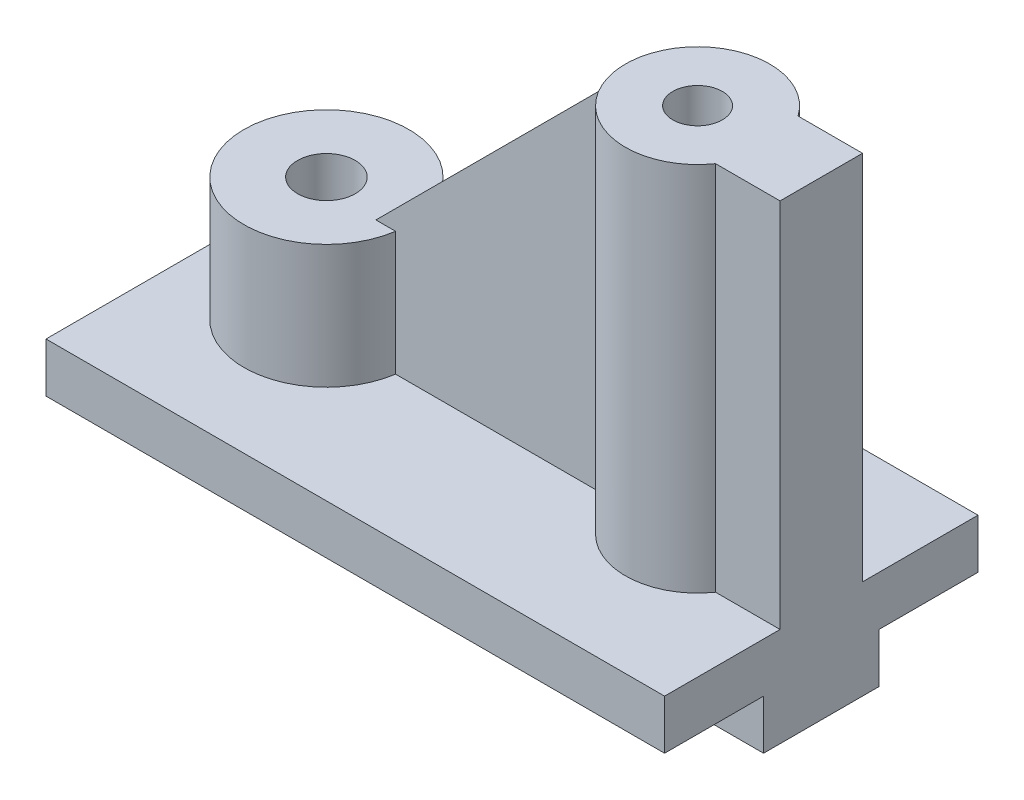
ISO-10303-21;
HEADER;
FILE_DESCRIPTION(('STEP AP214'),'2;1');
FILE_NAME('part.step','',(''),(''),'','','');
FILE_SCHEMA(('AUTOMOTIVE_DESIGN { 1 0 10303 214 1 1 1 1 }'));
ENDSEC;
DATA;
#1=APPLICATION_CONTEXT('core data for automotive mechanical design processes');
#2=APPLICATION_PROTOCOL_DEFINITION('international standard','automotive_design',2000,#1);
#3=PRODUCT_CONTEXT('',#1,'mechanical');
#4=PRODUCT('Part','Part','',(#3));
#5=PRODUCT_RELATED_PRODUCT_CATEGORY('part','',(#4));
#6=PRODUCT_DEFINITION_FORMATION('','',#4);
#7=PRODUCT_DEFINITION_CONTEXT('part definition',#1,'design');
#8=PRODUCT_DEFINITION('design','',#6,#7);
#9=PRODUCT_DEFINITION_SHAPE('','',#8);
#10=(LENGTH_UNIT() NAMED_UNIT(*) SI_UNIT(.MILLI.,.METRE.));
#11=(NAMED_UNIT(*) PLANE_ANGLE_UNIT() SI_UNIT($,.RADIAN.));
#12=(NAMED_UNIT(*) SI_UNIT($,.STERADIAN.) SOLID_ANGLE_UNIT());
#13=UNCERTAINTY_MEASURE_WITH_UNIT(LENGTH_MEASURE(1.E-05),#10,'distance_accuracy_value','');
#14=(GEOMETRIC_REPRESENTATION_CONTEXT(3) GLOBAL_UNCERTAINTY_ASSIGNED_CONTEXT((#13)) GLOBAL_UNIT_ASSIGNED_CONTEXT((#10,
#11,#12)) REPRESENTATION_CONTEXT('',''));
#15=CARTESIAN_POINT('',(0.,0.,0.));
#16=DIRECTION('',(0.,0.,1.));
#17=DIRECTION('',(1.,0.,0.));
#18=AXIS2_PLACEMENT_3D('',#15,#16,#17);
#19=CARTESIAN_POINT('',(0.,0.,-35.));
#20=DIRECTION('',(0.,0.,1.));
#21=DIRECTION('',(1.,0.,0.));
#22=AXIS2_PLACEMENT_3D('',#19,#20,#21);
#23=PLANE('',#22);
#24=DIRECTION('',(-1.,0.,0.));
#25=VECTOR('',#24,1.);
#26=CARTESIAN_POINT('',(0.,42.,-35.));
#27=LINE('',#26,#25);
#28=CARTESIAN_POINT('',(49.7737199332852,42.,-35.));
#29=VERTEX_POINT('',#28);
#30=CARTESIAN_POINT('',(45.,42.,-35.));
#31=VERTEX_POINT('',#30);
#32=EDGE_CURVE('E65',#29,#31,#27,.T.);
#33=ORIENTED_EDGE('',*,*,#32,.F.);
#34=DIRECTION('',(0.,-1.,0.));
#35=VECTOR('',#34,1.);
#36=CARTESIAN_POINT('',(49.7737199332852,42.,-35.));
#37=LINE('',#36,#35);
#38=CARTESIAN_POINT('',(49.7737199332852,12.,-35.));
#39=VERTEX_POINT('',#38);
#40=EDGE_CURVE('E286',#29,#39,#37,.T.);
#41=ORIENTED_EDGE('',*,*,#40,.T.);
#42=DIRECTION('',(1.,0.,0.));
#43=VECTOR('',#42,1.);
#44=CARTESIAN_POINT('',(45.,12.,-35.));
#45=LINE('',#44,#43);
#46=CARTESIAN_POINT('',(102.759060350433,12.,-35.));
#47=VERTEX_POINT('',#46);
#48=EDGE_CURVE('E266',#39,#47,#45,.T.);
#49=ORIENTED_EDGE('',*,*,#48,.T.);
#50=DIRECTION('',(0.,-1.,0.));
#51=VECTOR('',#50,1.);
#52=CARTESIAN_POINT('',(102.759060350433,102.,-35.));
#53=LINE('',#52,#51);
#54=CARTESIAN_POINT('',(102.759060350433,99.7590603504333,-35.));
#55=VERTEX_POINT('',#54);
#56=EDGE_CURVE('E268',#47,#55,#53,.F.);
#57=ORIENTED_EDGE('',*,*,#56,.T.);
#58=DIRECTION('',(-0.707106781186547,-0.707106781186548,0.));
#59=VECTOR('',#58,1.);
#60=CARTESIAN_POINT('',(105.,102.,-35.));
#61=LINE('',#60,#59);
#62=EDGE_CURVE('E265',#55,#31,#61,.T.);
#63=ORIENTED_EDGE('',*,*,#62,.T.);
#64=EDGE_LOOP('',(#33,#41,#49,#57,#63));
#65=FACE_BOUND('',#64,.T.);
#66=ADVANCED_FACE('F39',(#65),#23,.T.);
#67=CARTESIAN_POINT('',(0.,0.,-41.));
#68=DIRECTION('',(0.,0.,1.));
#69=DIRECTION('',(1.,0.,0.));
#70=AXIS2_PLACEMENT_3D('',#67,#68,#69);
#71=PLANE('',#70);
#72=DIRECTION('',(0.,-1.,0.));
#73=VECTOR('',#72,1.);
#74=CARTESIAN_POINT('',(49.7737199332852,42.,-41.));
#75=LINE('',#74,#73);
#76=CARTESIAN_POINT('',(49.7737199332852,42.,-41.));
#77=VERTEX_POINT('',#76);
#78=CARTESIAN_POINT('',(49.7737199332852,12.,-41.));
#79=VERTEX_POINT('',#78);
#80=EDGE_CURVE('E290',#77,#79,#75,.T.);
#81=ORIENTED_EDGE('',*,*,#80,.F.);
#82=DIRECTION('',(-1.,0.,0.));
#83=VECTOR('',#82,1.);
#84=CARTESIAN_POINT('',(0.,42.,-41.));
#85=LINE('',#84,#83);
#86=CARTESIAN_POINT('',(45.,42.,-41.));
#87=VERTEX_POINT('',#86);
#88=EDGE_CURVE('E295',#77,#87,#85,.T.);
#89=ORIENTED_EDGE('',*,*,#88,.T.);
#90=DIRECTION('',(-0.707106781186547,-0.707106781186548,0.));
#91=VECTOR('',#90,1.);
#92=CARTESIAN_POINT('',(105.,102.,-41.));
#93=LINE('',#92,#91);
#94=CARTESIAN_POINT('',(102.759060350433,99.7590603504333,-41.));
#95=VERTEX_POINT('',#94);
#96=EDGE_CURVE('E263',#95,#87,#93,.T.);
#97=ORIENTED_EDGE('',*,*,#96,.F.);
#98=DIRECTION('',(0.,-1.,0.));
#99=VECTOR('',#98,1.);
#100=CARTESIAN_POINT('',(102.759060350433,102.,-41.));
#101=LINE('',#100,#99);
#102=CARTESIAN_POINT('',(102.759060350433,12.,-41.));
#103=VERTEX_POINT('',#102);
#104=EDGE_CURVE('E11',#103,#95,#101,.F.);
#105=ORIENTED_EDGE('',*,*,#104,.F.);
#106=DIRECTION('',(1.,0.,0.));
#107=VECTOR('',#106,1.);
#108=CARTESIAN_POINT('',(75.,12.,-41.));
#109=LINE('',#108,#107);
#110=EDGE_CURVE('E267',#79,#103,#109,.T.);
#111=ORIENTED_EDGE('',*,*,#110,.F.);
#112=EDGE_LOOP('',(#81,#89,#97,#105,#111));
#113=FACE_BOUND('',#112,.T.);
#114=ADVANCED_FACE('F348',(#113),#71,.F.);
#115=CARTESIAN_POINT('',(105.,102.,-35.));
#116=DIRECTION('',(0.707106781186548,-0.707106781186547,0.));
#117=DIRECTION('',(0.707106781186547,0.707106781186548,0.));
#118=AXIS2_PLACEMENT_3D('',#115,#116,#117);
#119=PLANE('',#118);
#120=CARTESIAN_POINT('',(120.,117.,-38.));
#121=DIRECTION('',(0.707106781186548,-0.707106781186547,0.));
#122=DIRECTION('',(-0.707106781186547,-0.707106781186548,0.));
#123=AXIS2_PLACEMENT_3D('',#120,#121,#122);
#124=ELLIPSE('',#123,24.7487373415292,17.5);
#125=EDGE_CURVE('E271',#95,#55,#124,.F.);
#126=ORIENTED_EDGE('',*,*,#125,.F.);
#127=ORIENTED_EDGE('',*,*,#96,.T.);
#128=DIRECTION('',(0.,0.,-1.));
#129=VECTOR('',#128,1.);
#130=CARTESIAN_POINT('',(45.,42.,-35.));
#131=LINE('',#130,#129);
#132=EDGE_CURVE('E191',#31,#87,#131,.T.);
#133=ORIENTED_EDGE('',*,*,#132,.F.);
#134=ORIENTED_EDGE('',*,*,#62,.F.);
#135=EDGE_LOOP('',(#126,#127,#133,#134));
#136=FACE_BOUND('',#135,.T.);
#137=ADVANCED_FACE('F339',(#136),#119,.F.);
#138=CARTESIAN_POINT('',(150.,0.,-24.));
#139=DIRECTION('',(0.,1.,0.));
#140=DIRECTION('',(0.,0.,1.));
#141=AXIS2_PLACEMENT_3D('',#138,#139,#140);
#142=PLANE('',#141);
#143=DIRECTION('',(0.,0.,-1.));
#144=VECTOR('',#143,1.);
#145=CARTESIAN_POINT('',(0.,0.,-24.));
#146=LINE('',#145,#144);
#147=CARTESIAN_POINT('',(0.,0.,0.));
#148=VERTEX_POINT('',#147);
#149=CARTESIAN_POINT('',(0.,0.,-24.));
#150=VERTEX_POINT('',#149);
#151=EDGE_CURVE('E188',#148,#150,#146,.T.);
#152=ORIENTED_EDGE('',*,*,#151,.T.);
#153=DIRECTION('',(-1.,0.,0.));
#154=VECTOR('',#153,1.);
#155=CARTESIAN_POINT('',(150.,0.,-24.));
#156=LINE('',#155,#154);
#157=CARTESIAN_POINT('',(150.,0.,-24.));
#158=VERTEX_POINT('',#157);
#159=EDGE_CURVE('E50',#158,#150,#156,.T.);
#160=ORIENTED_EDGE('',*,*,#159,.F.);
#161=DIRECTION('',(0.,0.,-1.));
#162=VECTOR('',#161,1.);
#163=CARTESIAN_POINT('',(150.,0.,-24.));
#164=LINE('',#163,#162);
#165=CARTESIAN_POINT('',(150.,0.,0.));
#166=VERTEX_POINT('',#165);
#167=EDGE_CURVE('E206',#166,#158,#164,.T.);
#168=ORIENTED_EDGE('',*,*,#167,.F.);
#169=DIRECTION('',(-1.,0.,0.));
#170=VECTOR('',#169,1.);
#171=CARTESIAN_POINT('',(150.,0.,0.));
#172=LINE('',#171,#170);
#173=EDGE_CURVE('E184',#166,#148,#172,.T.);
#174=ORIENTED_EDGE('',*,*,#173,.T.);
#175=EDGE_LOOP('',(#152,#160,#168,#174));
#176=FACE_BOUND('',#175,.T.);
#177=ADVANCED_FACE('F41',(#176),#142,.F.);
#178=CARTESIAN_POINT('',(150.,-12.,-24.));
#179=DIRECTION('',(0.,0.,-1.));
#180=DIRECTION('',(-1.,0.,0.));
#181=AXIS2_PLACEMENT_3D('',#178,#179,#180);
#182=PLANE('',#181);
#183=DIRECTION('',(0.,-1.,0.));
#184=VECTOR('',#183,1.);
#185=CARTESIAN_POINT('',(0.,-12.,-24.));
#186=LINE('',#185,#184);
#187=CARTESIAN_POINT('',(0.,-12.,-24.));
#188=VERTEX_POINT('',#187);
#189=EDGE_CURVE('E194',#150,#188,#186,.T.);
#190=ORIENTED_EDGE('',*,*,#189,.T.);
#191=DIRECTION('',(-1.,0.,0.));
#192=VECTOR('',#191,1.);
#193=CARTESIAN_POINT('',(150.,-12.,-24.));
#194=LINE('',#193,#192);
#195=CARTESIAN_POINT('',(150.,-12.,-24.));
#196=VERTEX_POINT('',#195);
#197=EDGE_CURVE('E225',#196,#188,#194,.T.);
#198=ORIENTED_EDGE('',*,*,#197,.F.);
#199=DIRECTION('',(0.,-1.,0.));
#200=VECTOR('',#199,1.);
#201=CARTESIAN_POINT('',(150.,-12.,-24.));
#202=LINE('',#201,#200);
#203=EDGE_CURVE('E235',#158,#196,#202,.T.);
#204=ORIENTED_EDGE('',*,*,#203,.F.);
#205=ORIENTED_EDGE('',*,*,#159,.T.);
#206=EDGE_LOOP('',(#190,#198,#204,#205));
#207=FACE_BOUND('',#206,.T.);
#208=ADVANCED_FACE('F229',(#207),#182,.F.);
#209=CARTESIAN_POINT('',(150.,-12.,-52.));
#210=DIRECTION('',(0.,1.,0.));
#211=DIRECTION('',(0.,0.,1.));
#212=AXIS2_PLACEMENT_3D('',#209,#210,#211);
#213=PLANE('',#212);
#214=CARTESIAN_POINT('',(30.,-12.,-38.));
#215=DIRECTION('',(0.,1.,0.));
#216=DIRECTION('',(0.,0.,1.));
#217=AXIS2_PLACEMENT_3D('',#214,#215,#216);
#218=CIRCLE('',#217,7.);
#219=CARTESIAN_POINT('',(30.,-12.,-31.));
#220=VERTEX_POINT('',#219);
#221=EDGE_CURVE('E301',#220,#220,#218,.T.);
#222=ORIENTED_EDGE('',*,*,#221,.T.);
#223=EDGE_LOOP('',(#222));
#224=FACE_BOUND('',#223,.T.);
#225=CARTESIAN_POINT('',(120.,-12.,-38.));
#226=DIRECTION('',(0.,1.,0.));
#227=DIRECTION('',(0.,0.,1.));
#228=AXIS2_PLACEMENT_3D('',#225,#226,#227);
#229=CIRCLE('',#228,6.00000000000002);
#230=CARTESIAN_POINT('',(120.,-12.,-32.));
#231=VERTEX_POINT('',#230);
#232=EDGE_CURVE('E282',#231,#231,#229,.T.);
#233=ORIENTED_EDGE('',*,*,#232,.T.);
#234=EDGE_LOOP('',(#233));
#235=FACE_BOUND('',#234,.T.);
#236=DIRECTION('',(0.,0.,-1.));
#237=VECTOR('',#236,1.);
#238=CARTESIAN_POINT('',(0.,-12.,-52.));
#239=LINE('',#238,#237);
#240=CARTESIAN_POINT('',(0.,-12.,-52.));
#241=VERTEX_POINT('',#240);
#242=EDGE_CURVE('E199',#188,#241,#239,.T.);
#243=ORIENTED_EDGE('',*,*,#242,.T.);
#244=DIRECTION('',(-1.,0.,0.));
#245=VECTOR('',#244,1.);
#246=CARTESIAN_POINT('',(150.,-12.,-52.));
#247=LINE('',#246,#245);
#248=CARTESIAN_POINT('',(150.,-12.,-52.));
#249=VERTEX_POINT('',#248);
#250=EDGE_CURVE('E222',#249,#241,#247,.T.);
#251=ORIENTED_EDGE('',*,*,#250,.F.);
#252=DIRECTION('',(0.,0.,-1.));
#253=VECTOR('',#252,1.);
#254=CARTESIAN_POINT('',(150.,-12.,-52.));
#255=LINE('',#254,#253);
#256=EDGE_CURVE('E253',#196,#249,#255,.T.);
#257=ORIENTED_EDGE('',*,*,#256,.F.);
#258=ORIENTED_EDGE('',*,*,#197,.T.);
#259=EDGE_LOOP('',(#243,#251,#257,#258));
#260=FACE_BOUND('',#259,.T.);
#261=ADVANCED_FACE('F246',(#224,#235,#260),#213,.F.);
#262=CARTESIAN_POINT('',(150.,0.,-52.));
#263=DIRECTION('',(0.,0.,1.));
#264=DIRECTION('',(1.,0.,0.));
#265=AXIS2_PLACEMENT_3D('',#262,#263,#264);
#266=PLANE('',#265);
#267=DIRECTION('',(0.,1.,0.));
#268=VECTOR('',#267,1.);
#269=CARTESIAN_POINT('',(0.,0.,-52.));
#270=LINE('',#269,#268);
#271=CARTESIAN_POINT('',(0.,0.,-52.));
#272=VERTEX_POINT('',#271);
#273=EDGE_CURVE('E200',#241,#272,#270,.T.);
#274=ORIENTED_EDGE('',*,*,#273,.T.);
#275=DIRECTION('',(-1.,0.,0.));
#276=VECTOR('',#275,1.);
#277=CARTESIAN_POINT('',(150.,0.,-52.));
#278=LINE('',#277,#276);
#279=CARTESIAN_POINT('',(150.,0.,-52.));
#280=VERTEX_POINT('',#279);
#281=EDGE_CURVE('E218',#280,#272,#278,.T.);
#282=ORIENTED_EDGE('',*,*,#281,.F.);
#283=DIRECTION('',(0.,1.,0.));
#284=VECTOR('',#283,1.);
#285=CARTESIAN_POINT('',(150.,0.,-52.));
#286=LINE('',#285,#284);
#287=EDGE_CURVE('E255',#249,#280,#286,.T.);
#288=ORIENTED_EDGE('',*,*,#287,.F.);
#289=ORIENTED_EDGE('',*,*,#250,.T.);
#290=EDGE_LOOP('',(#274,#282,#288,#289));
#291=FACE_BOUND('',#290,.T.);
#292=ADVANCED_FACE('F249',(#291),#266,.F.);
#293=CARTESIAN_POINT('',(150.,0.,-76.));
#294=DIRECTION('',(0.,1.,0.));
#295=DIRECTION('',(0.,0.,1.));
#296=AXIS2_PLACEMENT_3D('',#293,#294,#295);
#297=PLANE('',#296);
#298=DIRECTION('',(0.,0.,-1.));
#299=VECTOR('',#298,1.);
#300=CARTESIAN_POINT('',(0.,0.,-76.));
#301=LINE('',#300,#299);
#302=CARTESIAN_POINT('',(0.,0.,-76.));
#303=VERTEX_POINT('',#302);
#304=EDGE_CURVE('E197',#272,#303,#301,.T.);
#305=ORIENTED_EDGE('',*,*,#304,.T.);
#306=DIRECTION('',(-1.,0.,0.));
#307=VECTOR('',#306,1.);
#308=CARTESIAN_POINT('',(150.,0.,-76.));
#309=LINE('',#308,#307);
#310=CARTESIAN_POINT('',(150.,0.,-76.));
#311=VERTEX_POINT('',#310);
#312=EDGE_CURVE('E219',#311,#303,#309,.T.);
#313=ORIENTED_EDGE('',*,*,#312,.F.);
#314=DIRECTION('',(0.,0.,-1.));
#315=VECTOR('',#314,1.);
#316=CARTESIAN_POINT('',(150.,0.,-76.));
#317=LINE('',#316,#315);
#318=EDGE_CURVE('E251',#280,#311,#317,.T.);
#319=ORIENTED_EDGE('',*,*,#318,.F.);
#320=ORIENTED_EDGE('',*,*,#281,.T.);
#321=EDGE_LOOP('',(#305,#313,#319,#320));
#322=FACE_BOUND('',#321,.T.);
#323=ADVANCED_FACE('F373',(#322),#297,.F.);
#324=CARTESIAN_POINT('',(150.,12.,-76.));
#325=DIRECTION('',(0.,0.,1.));
#326=DIRECTION('',(1.,0.,0.));
#327=AXIS2_PLACEMENT_3D('',#324,#325,#326);
#328=PLANE('',#327);
#329=DIRECTION('',(0.,1.,0.));
#330=VECTOR('',#329,1.);
#331=CARTESIAN_POINT('',(0.,12.,-76.));
#332=LINE('',#331,#330);
#333=CARTESIAN_POINT('',(0.,12.,-76.));
#334=VERTEX_POINT('',#333);
#335=EDGE_CURVE('E202',#303,#334,#332,.T.);
#336=ORIENTED_EDGE('',*,*,#335,.T.);
#337=DIRECTION('',(-1.,0.,0.));
#338=VECTOR('',#337,1.);
#339=CARTESIAN_POINT('',(150.,12.,-76.));
#340=LINE('',#339,#338);
#341=CARTESIAN_POINT('',(150.,12.,-76.));
#342=VERTEX_POINT('',#341);
#343=EDGE_CURVE('E211',#342,#334,#340,.T.);
#344=ORIENTED_EDGE('',*,*,#343,.F.);
#345=DIRECTION('',(0.,1.,0.));
#346=VECTOR('',#345,1.);
#347=CARTESIAN_POINT('',(150.,12.,-76.));
#348=LINE('',#347,#346);
#349=EDGE_CURVE('E179',#311,#342,#348,.T.);
#350=ORIENTED_EDGE('',*,*,#349,.F.);
#351=ORIENTED_EDGE('',*,*,#312,.T.);
#352=EDGE_LOOP('',(#336,#344,#350,#351));
#353=FACE_BOUND('',#352,.T.);
#354=ADVANCED_FACE('F369',(#353),#328,.F.);
#355=CARTESIAN_POINT('',(150.,12.,0.));
#356=DIRECTION('',(0.,-1.,0.));
#357=DIRECTION('',(0.,0.,-1.));
#358=AXIS2_PLACEMENT_3D('',#355,#356,#357);
#359=PLANE('',#358);
#360=DIRECTION('',(0.,0.,1.));
#361=VECTOR('',#360,1.);
#362=CARTESIAN_POINT('',(150.,12.,0.));
#363=LINE('',#362,#361);
#364=CARTESIAN_POINT('',(150.,12.,-28.));
#365=VERTEX_POINT('',#364);
#366=CARTESIAN_POINT('',(150.,12.,0.));
#367=VERTEX_POINT('',#366);
#368=EDGE_CURVE('E182',#365,#367,#363,.T.);
#369=ORIENTED_EDGE('',*,*,#368,.F.);
#370=DIRECTION('',(1.,0.,0.));
#371=VECTOR('',#370,1.);
#372=CARTESIAN_POINT('',(130.,12.,-28.));
#373=LINE('',#372,#371);
#374=CARTESIAN_POINT('',(134.361406616345,12.,-28.));
#375=VERTEX_POINT('',#374);
#376=EDGE_CURVE('E312',#375,#365,#373,.T.);
#377=ORIENTED_EDGE('',*,*,#376,.F.);
#378=CARTESIAN_POINT('',(120.,12.,-38.));
#379=DIRECTION('',(0.,1.,0.));
#380=DIRECTION('',(0.,0.,1.));
#381=AXIS2_PLACEMENT_3D('',#378,#379,#380);
#382=CIRCLE('',#381,17.5);
#383=EDGE_CURVE('E280',#47,#375,#382,.T.);
#384=ORIENTED_EDGE('',*,*,#383,.F.);
#385=ORIENTED_EDGE('',*,*,#48,.F.);
#386=CARTESIAN_POINT('',(30.,12.,-38.));
#387=DIRECTION('',(0.,1.,0.));
#388=DIRECTION('',(0.,0.,1.));
#389=AXIS2_PLACEMENT_3D('',#386,#387,#388);
#390=CIRCLE('',#389,20.);
#391=EDGE_CURVE('E296',#79,#39,#390,.T.);
#392=ORIENTED_EDGE('',*,*,#391,.F.);
#393=ORIENTED_EDGE('',*,*,#110,.T.);
#394=CARTESIAN_POINT('',(134.361406616345,12.,-48.));
#395=VERTEX_POINT('',#394);
#396=EDGE_CURVE('E172',#395,#103,#382,.T.);
#397=ORIENTED_EDGE('',*,*,#396,.F.);
#398=DIRECTION('',(1.,0.,0.));
#399=VECTOR('',#398,1.);
#400=CARTESIAN_POINT('',(130.,12.,-48.));
#401=LINE('',#400,#399);
#402=CARTESIAN_POINT('',(150.,12.,-48.));
#403=VERTEX_POINT('',#402);
#404=EDGE_CURVE('E53',#395,#403,#401,.T.);
#405=ORIENTED_EDGE('',*,*,#404,.T.);
#406=EDGE_CURVE('E175',#342,#403,#363,.T.);
#407=ORIENTED_EDGE('',*,*,#406,.F.);
#408=ORIENTED_EDGE('',*,*,#343,.T.);
#409=DIRECTION('',(0.,0.,1.));
#410=VECTOR('',#409,1.);
#411=CARTESIAN_POINT('',(0.,12.,0.));
#412=LINE('',#411,#410);
#413=CARTESIAN_POINT('',(0.,12.,0.));
#414=VERTEX_POINT('',#413);
#415=EDGE_CURVE('E203',#334,#414,#412,.T.);
#416=ORIENTED_EDGE('',*,*,#415,.T.);
#417=DIRECTION('',(-1.,0.,0.));
#418=VECTOR('',#417,1.);
#419=CARTESIAN_POINT('',(150.,12.,0.));
#420=LINE('',#419,#418);
#421=EDGE_CURVE('E212',#367,#414,#420,.T.);
#422=ORIENTED_EDGE('',*,*,#421,.F.);
#423=EDGE_LOOP('',(#369,#377,#384,#385,#392,#393,#397,#405,#407,#408,#416,#422));
#424=FACE_BOUND('',#423,.T.);
#425=ADVANCED_FACE('F167',(#424),#359,.F.);
#426=CARTESIAN_POINT('',(150.,0.,0.));
#427=DIRECTION('',(0.,0.,-1.));
#428=DIRECTION('',(-1.,0.,0.));
#429=AXIS2_PLACEMENT_3D('',#426,#427,#428);
#430=PLANE('',#429);
#431=DIRECTION('',(0.,-1.,0.));
#432=VECTOR('',#431,1.);
#433=CARTESIAN_POINT('',(0.,0.,0.));
#434=LINE('',#433,#432);
#435=EDGE_CURVE('E207',#414,#148,#434,.T.);
#436=ORIENTED_EDGE('',*,*,#435,.T.);
#437=ORIENTED_EDGE('',*,*,#173,.F.);
#438=DIRECTION('',(0.,-1.,0.));
#439=VECTOR('',#438,1.);
#440=CARTESIAN_POINT('',(150.,0.,0.));
#441=LINE('',#440,#439);
#442=EDGE_CURVE('E185',#367,#166,#441,.T.);
#443=ORIENTED_EDGE('',*,*,#442,.F.);
#444=ORIENTED_EDGE('',*,*,#421,.T.);
#445=EDGE_LOOP('',(#436,#437,#443,#444));
#446=FACE_BOUND('',#445,.T.);
#447=ADVANCED_FACE('F365',(#446),#430,.F.);
#448=CARTESIAN_POINT('',(150.,0.,0.));
#449=DIRECTION('',(-1.,0.,0.));
#450=DIRECTION('',(0.,0.,1.));
#451=AXIS2_PLACEMENT_3D('',#448,#449,#450);
#452=PLANE('',#451);
#453=ORIENTED_EDGE('',*,*,#167,.T.);
#454=ORIENTED_EDGE('',*,*,#203,.T.);
#455=ORIENTED_EDGE('',*,*,#256,.T.);
#456=ORIENTED_EDGE('',*,*,#287,.T.);
#457=ORIENTED_EDGE('',*,*,#318,.T.);
#458=ORIENTED_EDGE('',*,*,#349,.T.);
#459=ORIENTED_EDGE('',*,*,#406,.T.);
#460=DIRECTION('',(0.,1.,0.));
#461=VECTOR('',#460,1.);
#462=CARTESIAN_POINT('',(150.,102.,-48.));
#463=LINE('',#462,#461);
#464=CARTESIAN_POINT('',(150.,102.,-48.));
#465=VERTEX_POINT('',#464);
#466=EDGE_CURVE('E156',#403,#465,#463,.T.);
#467=ORIENTED_EDGE('',*,*,#466,.T.);
#468=DIRECTION('',(0.,0.,1.));
#469=VECTOR('',#468,1.);
#470=CARTESIAN_POINT('',(150.,102.,-28.));
#471=LINE('',#470,#469);
#472=CARTESIAN_POINT('',(150.,102.,-28.));
#473=VERTEX_POINT('',#472);
#474=EDGE_CURVE('E165',#465,#473,#471,.T.);
#475=ORIENTED_EDGE('',*,*,#474,.T.);
#476=DIRECTION('',(0.,-1.,0.));
#477=VECTOR('',#476,1.);
#478=CARTESIAN_POINT('',(150.,12.,-28.));
#479=LINE('',#478,#477);
#480=EDGE_CURVE('E174',#473,#365,#479,.T.);
#481=ORIENTED_EDGE('',*,*,#480,.T.);
#482=ORIENTED_EDGE('',*,*,#368,.T.);
#483=ORIENTED_EDGE('',*,*,#442,.T.);
#484=EDGE_LOOP('',(#453,#454,#455,#456,#457,#458,#459,#467,#475,#481,#482,#483));
#485=FACE_BOUND('',#484,.T.);
#486=ADVANCED_FACE('F178',(#485),#452,.F.);
#487=CARTESIAN_POINT('',(0.,0.,0.));
#488=DIRECTION('',(-1.,0.,0.));
#489=DIRECTION('',(0.,0.,1.));
#490=AXIS2_PLACEMENT_3D('',#487,#488,#489);
#491=PLANE('',#490);
#492=ORIENTED_EDGE('',*,*,#151,.F.);
#493=ORIENTED_EDGE('',*,*,#435,.F.);
#494=ORIENTED_EDGE('',*,*,#415,.F.);
#495=ORIENTED_EDGE('',*,*,#335,.F.);
#496=ORIENTED_EDGE('',*,*,#304,.F.);
#497=ORIENTED_EDGE('',*,*,#273,.F.);
#498=ORIENTED_EDGE('',*,*,#242,.F.);
#499=ORIENTED_EDGE('',*,*,#189,.F.);
#500=EDGE_LOOP('',(#492,#493,#494,#495,#496,#497,#498,#499));
#501=FACE_BOUND('',#500,.T.);
#502=ADVANCED_FACE('F237',(#501),#491,.T.);
#503=CARTESIAN_POINT('',(120.,102.,-38.));
#504=DIRECTION('',(0.,-1.,0.));
#505=DIRECTION('',(0.,0.,-1.));
#506=AXIS2_PLACEMENT_3D('',#503,#504,#505);
#507=CYLINDRICAL_SURFACE('',#506,17.5);
#508=ORIENTED_EDGE('',*,*,#383,.T.);
#509=DIRECTION('',(0.,-1.,0.));
#510=VECTOR('',#509,1.);
#511=CARTESIAN_POINT('',(134.361406616345,102.,-28.));
#512=LINE('',#511,#510);
#513=CARTESIAN_POINT('',(134.361406616345,102.,-28.));
#514=VERTEX_POINT('',#513);
#515=EDGE_CURVE('E310',#375,#514,#512,.F.);
#516=ORIENTED_EDGE('',*,*,#515,.T.);
#517=CARTESIAN_POINT('',(120.,102.,-38.));
#518=DIRECTION('',(0.,1.,0.));
#519=DIRECTION('',(0.,0.,1.));
#520=AXIS2_PLACEMENT_3D('',#517,#518,#519);
#521=CIRCLE('',#520,17.5);
#522=CARTESIAN_POINT('',(134.361406616345,102.,-48.));
#523=VERTEX_POINT('',#522);
#524=EDGE_CURVE('E277',#523,#514,#521,.T.);
#525=ORIENTED_EDGE('',*,*,#524,.F.);
#526=DIRECTION('',(0.,-1.,0.));
#527=VECTOR('',#526,1.);
#528=CARTESIAN_POINT('',(134.361406616345,102.,-48.));
#529=LINE('',#528,#527);
#530=EDGE_CURVE('E315',#523,#395,#529,.T.);
#531=ORIENTED_EDGE('',*,*,#530,.T.);
#532=ORIENTED_EDGE('',*,*,#396,.T.);
#533=ORIENTED_EDGE('',*,*,#104,.T.);
#534=ORIENTED_EDGE('',*,*,#125,.T.);
#535=ORIENTED_EDGE('',*,*,#56,.F.);
#536=EDGE_LOOP('',(#508,#516,#525,#531,#532,#533,#534,#535));
#537=FACE_BOUND('',#536,.T.);
#538=ADVANCED_FACE('F333',(#537),#507,.T.);
#539=CARTESIAN_POINT('',(120.,102.,-38.));
#540=DIRECTION('',(0.,1.,0.));
#541=DIRECTION('',(0.,0.,1.));
#542=AXIS2_PLACEMENT_3D('',#539,#540,#541);
#543=PLANE('',#542);
#544=ORIENTED_EDGE('',*,*,#524,.T.);
#545=DIRECTION('',(1.,0.,0.));
#546=VECTOR('',#545,1.);
#547=CARTESIAN_POINT('',(130.,102.,-28.));
#548=LINE('',#547,#546);
#549=EDGE_CURVE('E317',#514,#473,#548,.T.);
#550=ORIENTED_EDGE('',*,*,#549,.T.);
#551=ORIENTED_EDGE('',*,*,#474,.F.);
#552=DIRECTION('',(1.,0.,0.));
#553=VECTOR('',#552,1.);
#554=CARTESIAN_POINT('',(130.,102.,-48.));
#555=LINE('',#554,#553);
#556=EDGE_CURVE('E158',#523,#465,#555,.T.);
#557=ORIENTED_EDGE('',*,*,#556,.F.);
#558=EDGE_LOOP('',(#544,#550,#551,#557));
#559=FACE_BOUND('',#558,.T.);
#560=CARTESIAN_POINT('',(120.,102.,-38.));
#561=DIRECTION('',(0.,1.,0.));
#562=DIRECTION('',(0.,0.,1.));
#563=AXIS2_PLACEMENT_3D('',#560,#561,#562);
#564=CIRCLE('',#563,6.00000000000002);
#565=CARTESIAN_POINT('',(120.,102.,-32.));
#566=VERTEX_POINT('',#565);
#567=EDGE_CURVE('E281',#566,#566,#564,.T.);
#568=ORIENTED_EDGE('',*,*,#567,.F.);
#569=EDGE_LOOP('',(#568));
#570=FACE_BOUND('',#569,.T.);
#571=ADVANCED_FACE('F324',(#559,#570),#543,.T.);
#572=CARTESIAN_POINT('',(120.,-12.,-38.));
#573=DIRECTION('',(0.,1.,0.));
#574=DIRECTION('',(0.,0.,1.));
#575=AXIS2_PLACEMENT_3D('',#572,#573,#574);
#576=CYLINDRICAL_SURFACE('',#575,6.00000000000002);
#577=ORIENTED_EDGE('',*,*,#232,.F.);
#578=EDGE_LOOP('',(#577));
#579=FACE_BOUND('',#578,.T.);
#580=ORIENTED_EDGE('',*,*,#567,.T.);
#581=EDGE_LOOP('',(#580));
#582=FACE_BOUND('',#581,.T.);
#583=ADVANCED_FACE('F468',(#579,#582),#576,.F.);
#584=CARTESIAN_POINT('',(30.,42.,-38.));
#585=DIRECTION('',(0.,-1.,0.));
#586=DIRECTION('',(0.,0.,-1.));
#587=AXIS2_PLACEMENT_3D('',#584,#585,#586);
#588=CYLINDRICAL_SURFACE('',#587,20.);
#589=ORIENTED_EDGE('',*,*,#40,.F.);
#590=CARTESIAN_POINT('',(30.,42.,-38.));
#591=DIRECTION('',(0.,1.,0.));
#592=DIRECTION('',(0.,0.,1.));
#593=AXIS2_PLACEMENT_3D('',#590,#591,#592);
#594=CIRCLE('',#593,20.);
#595=EDGE_CURVE('E300',#77,#29,#594,.T.);
#596=ORIENTED_EDGE('',*,*,#595,.F.);
#597=ORIENTED_EDGE('',*,*,#80,.T.);
#598=ORIENTED_EDGE('',*,*,#391,.T.);
#599=EDGE_LOOP('',(#589,#596,#597,#598));
#600=FACE_BOUND('',#599,.T.);
#601=ADVANCED_FACE('F343',(#600),#588,.T.);
#602=CARTESIAN_POINT('',(30.,42.,-38.));
#603=DIRECTION('',(0.,1.,0.));
#604=DIRECTION('',(0.,0.,1.));
#605=AXIS2_PLACEMENT_3D('',#602,#603,#604);
#606=PLANE('',#605);
#607=CARTESIAN_POINT('',(30.,42.,-38.));
#608=DIRECTION('',(0.,1.,0.));
#609=DIRECTION('',(0.,0.,1.));
#610=AXIS2_PLACEMENT_3D('',#607,#608,#609);
#611=CIRCLE('',#610,7.);
#612=CARTESIAN_POINT('',(30.,42.,-31.));
#613=VERTEX_POINT('',#612);
#614=EDGE_CURVE('E302',#613,#613,#611,.T.);
#615=ORIENTED_EDGE('',*,*,#614,.F.);
#616=EDGE_LOOP('',(#615));
#617=FACE_BOUND('',#616,.T.);
#618=ORIENTED_EDGE('',*,*,#595,.T.);
#619=ORIENTED_EDGE('',*,*,#32,.T.);
#620=ORIENTED_EDGE('',*,*,#132,.T.);
#621=ORIENTED_EDGE('',*,*,#88,.F.);
#622=EDGE_LOOP('',(#618,#619,#620,#621));
#623=FACE_BOUND('',#622,.T.);
#624=ADVANCED_FACE('F345',(#617,#623),#606,.T.);
#625=CARTESIAN_POINT('',(30.,-12.,-38.));
#626=DIRECTION('',(0.,1.,0.));
#627=DIRECTION('',(0.,0.,1.));
#628=AXIS2_PLACEMENT_3D('',#625,#626,#627);
#629=CYLINDRICAL_SURFACE('',#628,7.);
#630=ORIENTED_EDGE('',*,*,#221,.F.);
#631=EDGE_LOOP('',(#630));
#632=FACE_BOUND('',#631,.T.);
#633=ORIENTED_EDGE('',*,*,#614,.T.);
#634=EDGE_LOOP('',(#633));
#635=FACE_BOUND('',#634,.T.);
#636=ADVANCED_FACE('F502',(#632,#635),#629,.F.);
#637=CARTESIAN_POINT('',(130.,12.,-28.));
#638=DIRECTION('',(0.,0.,1.));
#639=DIRECTION('',(1.,0.,0.));
#640=AXIS2_PLACEMENT_3D('',#637,#638,#639);
#641=PLANE('',#640);
#642=ORIENTED_EDGE('',*,*,#515,.F.);
#643=ORIENTED_EDGE('',*,*,#376,.T.);
#644=ORIENTED_EDGE('',*,*,#480,.F.);
#645=ORIENTED_EDGE('',*,*,#549,.F.);
#646=EDGE_LOOP('',(#642,#643,#644,#645));
#647=FACE_BOUND('',#646,.T.);
#648=ADVANCED_FACE('F326',(#647),#641,.T.);
#649=CARTESIAN_POINT('',(130.,102.,-48.));
#650=DIRECTION('',(0.,0.,-1.));
#651=DIRECTION('',(0.,1.,0.));
#652=AXIS2_PLACEMENT_3D('',#649,#650,#651);
#653=PLANE('',#652);
#654=ORIENTED_EDGE('',*,*,#530,.F.);
#655=ORIENTED_EDGE('',*,*,#556,.T.);
#656=ORIENTED_EDGE('',*,*,#466,.F.);
#657=ORIENTED_EDGE('',*,*,#404,.F.);
#658=EDGE_LOOP('',(#654,#655,#656,#657));
#659=FACE_BOUND('',#658,.T.);
#660=ADVANCED_FACE('F157',(#659),#653,.T.);
#661=CLOSED_SHELL('',(#66,#114,#137,#177,#208,#261,#292,#323,#354,#425,#447,#486,#502,#538,#571,
#583,#601,#624,#636,#648,#660));
#662=MANIFOLD_SOLID_BREP('B2',#661);
#663=ADVANCED_BREP_SHAPE_REPRESENTATION('',(#18,#662),#14);
#664=SHAPE_DEFINITION_REPRESENTATION(#9,#663);
ENDSEC;
END-ISO-10303-21;
